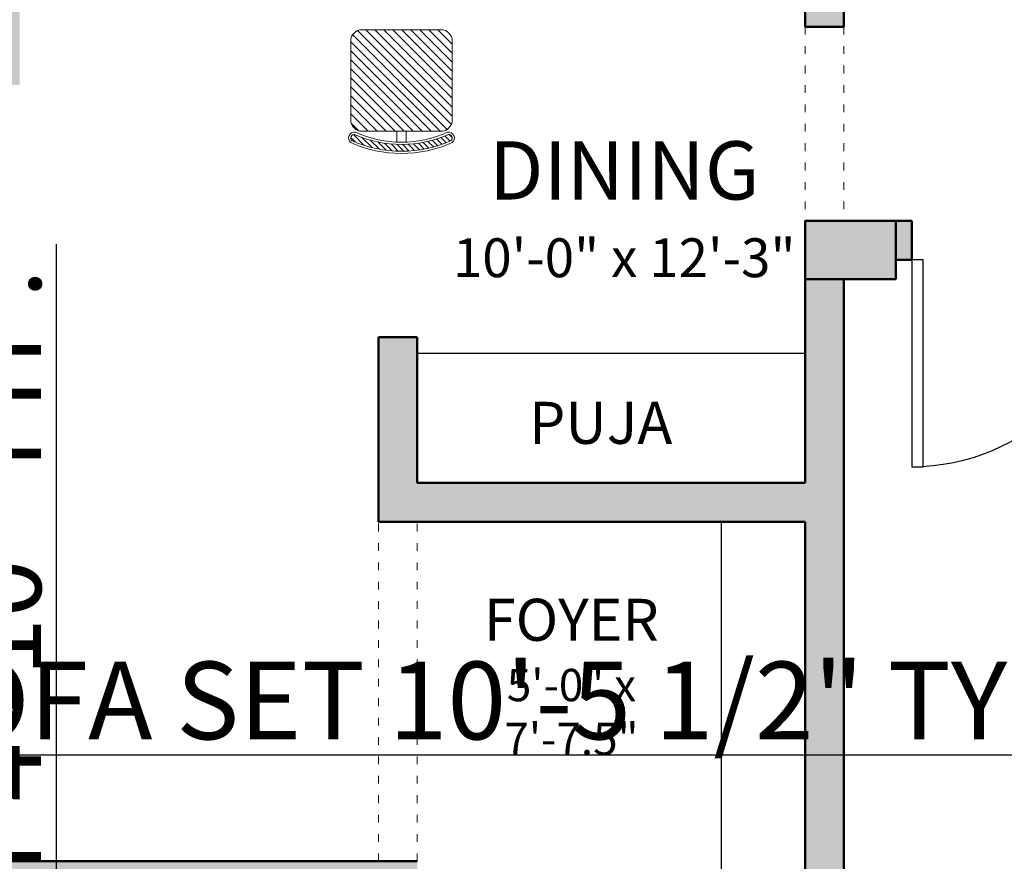
# Model space of a CAD drawing. Units: inches. Extents: x 375 to 1122, y 27 to 1069.
# Tile 83 of 155: x 667 to 819, y 716 to 846. Entities that reach past the tile are written whole.
import ezdxf

# ---------------------------------------------------------------- set-up
doc = ezdxf.new("R2010")
doc.units = ezdxf.units.IN
doc.linetypes.add('ACAD_ISO03W100', pattern=[30, 12, -18])
for name, color, linetype, lineweight in [('A-ANNO-DIMS', 2, 'Continuous', 18), ('A-AREA-IDEN', 7, 'Continuous', 18), ('A-COLS-PATT', 10, 'Continuous', 13), ('A-FLOR-MILL', 55, 'Continuous', 25), ('A-WALL-OVHD', 77, 'ACAD_ISO03W100', 18), ('A-WALL-PATT', 252, 'Continuous', 13), ('Columns', 10, 'Continuous', 50), ('Doors', 150, 'Continuous', 25), ('Furniture', 30, 'Continuous', 18), ('Walls', 250, 'Continuous', 50)]:
    doc.layers.add(name, color=color, linetype=linetype, lineweight=lineweight)
doc.styles.get("Standard").update_dxf_attribs({"font": 'arial.ttf'})
doc.dimstyles.new('ISO-25', dxfattribs={"dimtxt": 12, "dimasz": 2.5, "dimexe": 1.5, "dimexo": 1.5, "dimtad": 1, "dimdec": 1, "dimlunit": 3, "dimtxsty": 'Standard', "dimblk": 'ARCHTICK', "dimcen": 2.5, "dimadec": 0, "dimazin": 0, "dimtfac": 1, "dimtdec": 1, "dimtmove": 0, "dimatfit": 3, "dimfxl": 1.5, "dimfxlon": 1, "dimarcsym": 0})

# ---------------------------------------------------------------- blocks, each defined once
blk = doc.blocks.new('*U2')
for p, q in [((0, 0), (0, 4)), ((32, 0), (32, 4))]:
    blk.add_line(p, q)
blk.add_lwpolyline([(0, 0), (0, -32), (1.75, -32), (1.75, 0)], close=True)
blk.add_arc((0, 0), 32, 270, 0)
blk = doc.blocks.new('A$C403C54AD')
at = {"ltscale": 0.05}
for p, q in [((2.6911, 1.212, -0.0006), (2.3564, 0.8773, -0.0006)), ((2.6563, 1.212, -0.0006), (2.3564, 0.9121, -0.0006)), ((2.6215, 1.212, -0.0006), (2.3564, 0.9469, -0.0006)), ((2.5866, 1.212, -0.0006), (2.3564, 0.9818, -0.0006)), ((2.5518, 1.212, -0.0006), (2.3564, 1.0166, -0.0006)), ((2.517, 1.212, -0.0006), (2.3564, 1.0514, -0.0006)), ((2.4821, 1.212, -0.0006), (2.3564, 1.0862, -0.0006)), ((2.4473, 1.212, -0.0006), (2.3564, 1.1211, -0.0006)), ((2.4125, 1.212, -0.0006), (2.3564, 1.1559, -0.0006)), ((2.7225, 1.2085, -0.0006), (2.3599, 0.8459, -0.0006)), ((2.7416, 1.1928, -0.0006), (2.3756, 0.8268, -0.0006)), ((2.7734, 1.2115, -0.0006), (2.7615, 1.1996, -0.0006)), ((2.787, 1.2034, -0.0006), (2.767, 1.1834, -0.0006)), ((2.7934, 1.188, -0.0006), (2.7731, 1.1677, -0.0006)), ((2.7491, 1.1655, -0.0006), (2.4029, 0.8193, -0.0006)), ((2.7993, 1.1722, -0.0006), (2.7787, 1.1515, -0.0006)), ((2.8048, 1.1558, -0.0006), (2.7837, 1.1348, -0.0006)), ((2.7491, 1.1306, -0.0006), (2.4378, 0.8193, -0.0006)), ((2.8097, 1.139, -0.0006), (2.7882, 1.1175, -0.0006)), ((2.8141, 1.1216, -0.0006), (2.792, 1.0996, -0.0006)), ((2.7491, 1.0958, -0.0006), (2.4726, 0.8193, -0.0006)), ((2.8179, 1.1037, -0.0006), (2.7952, 1.081, -0.0006)), ((2.8211, 1.0851, -0.0006), (2.7977, 1.0617, -0.0006)), ((2.7491, 1.061, -0.0006), (2.5074, 0.8193, -0.0006)), ((2.8236, 1.0658, -0.0006), (2.7993, 1.0415, -0.0006)), ((2.8253, 1.0457, -0.0006), (2.8, 1.0205, -0.0006)), ((2.7491, 1.0262, -0.0006), (2.5422, 0.8193, -0.0006)), ((2.7491, 0.9913, -0.0006), (2.5771, 0.8193, -0.0006)), ((2.8261, 1.003, -0.0006), (2.7982, 0.9751, -0.0006)), ((2.8262, 1.0248, -0.0006), (2.7997, 0.9984, -0.0006)), ((2.7491, 0.9565, -0.0006), (2.6119, 0.8193, -0.0006)), ((2.8224, 0.9558, -0.0006), (2.7904, 0.9238, -0.0006)), ((2.8249, 0.98, -0.0006), (2.7952, 0.9504, -0.0006)), ((2.7491, 0.9217, -0.0006), (2.6467, 0.8193, -0.0006)), ((2.8184, 0.93, -0.0006), (2.7833, 0.8949, -0.0006)), ((2.7491, 0.8868, -0.0006), (2.6815, 0.8193, -0.0006)), ((2.8123, 0.9022, -0.0006), (2.7728, 0.8626, -0.0006)), ((2.7472, 0.8501, -0.0006), (2.7183, 0.8212, -0.0006)), ((2.8036, 0.8717, -0.0006), (2.7618, 0.8298, -0.0006)), ((2.791, 0.8373, -0.0006), (2.7733, 0.8196, -0.0006))]:
    blk.add_line(p, q, dxfattribs=at)
for p, q in [((2.7055, 1.212, -0.0006), (2.4001, 1.212, -0.0006)), ((2.3564, 1.1683, -0.0006), (2.3564, 0.8629, -0.0006)), ((2.7491, 0.8629, -0.0006), (2.7491, 1.1683, -0.0006)), ((2.7491, 1.0331, -0.0006), (2.7913, 1.0331, -0.0006)), ((2.7491, 0.9982, -0.0006), (2.7913, 0.9982, -0.0006)), ((2.4001, 0.8193, -0.0006), (2.531, 0.8193, -0.0006)), ((2.531, 0.8193, -0.0006), (2.7055, 0.8193, -0.0006))]:
    blk.add_line(p, q)
for centre, radius, start, end in [((2.7752, 1.1978, -0.0006), 0.0225, 38.8964, 189.6684), ((2.4001, 1.1683, -0.0006), 0.0436, 90, 180), ((2.7055, 1.1683, -0.0006), 0.0436, 0, 90), ((2.3575, 1.0156, -0.0006), 0.4338, 335.7176, 24.2824), ((2.3575, 1.0156, -0.0006), 0.4425, 335.7176, 24.2824), ((2.7752, 1.1978, -0.0006), 0.0138, 38.8964, 189.6684), ((2.3575, 1.0156, -0.0006), 0.4687, 335.7176, 24.2824), ((2.3575, 1.0156, -0.0006), 0.4774, 335.7176, 24.2824), ((2.4001, 0.8629, -0.0006), 0.0436, 180, 270), ((2.7055, 0.8629, -0.0006), 0.0436, 270, 0), ((2.7751, 0.8332, -0.0006), 0.0225, 169.7658, 321.6694), ((2.7751, 0.8332, -0.0006), 0.0138, 169.7658, 321.6694)]:
    blk.add_arc(centre, radius, start, end)
blk = doc.blocks.new('COLUMN-14X9IN')
blk.add_lwpolyline([(0, 0), (14, 0), (14, 9), (0, 9)], close=True)
blk = doc.blocks.new('_ArchTick')
at = {"color": 0, "linetype": 'ByBlock', "const_width": 0.15}
blk.add_lwpolyline([(-0.5, -0.5), (0.5, 0.5)], dxfattribs=at)
blk = doc.blocks.new('*D57')
at = {"layer": 'A-ANNO-DIMS', "color": 0, "lineweight": -2, "transparency": 16777216}
for p, q in [((512.46, 733.49), (512.46, 730.49)), ((638.07, 733.49), (638.07, 730.49)), ((512.46, 731.99), (638.07, 731.99)), ((638.07, 731.99), (839.76, 731.99))]:
    blk.add_line(p, q, dxfattribs=at)
at = {"layer": 'Defpoints', "color": 0, "transparency": 16777216}
for p in [(512.46, 750.84), (638.07, 750.84), (638.07, 731.99)]:
    blk.add_point(p, dxfattribs=at)
at = {"layer": 'A-ANNO-DIMS', "color": 0, "lineweight": -2, "transparency": 16777216, "xscale": 2.5, "yscale": 2.5, "zscale": 2.5, "rotation": 180}
blk.add_blockref('_ArchTick', (512.46, 731.99), dxfattribs=at)
at = {"layer": 'A-ANNO-DIMS', "color": 0, "lineweight": -2, "transparency": 16777216, "xscale": 2.5, "yscale": 2.5, "zscale": 2.5}
blk.add_blockref('_ArchTick', (638.07, 731.99), dxfattribs=at)
at = {"layer": 'A-ANNO-DIMS', "color": 0, "transparency": 16777216, "insert": (740.16, 738.83), "char_height": 12, "attachment_point": 5}
blk.add_mtext('SOFA SET 10\'-5 1/2" TYP.', dxfattribs=at)
blk = doc.blocks.new('*D58')
at = {"layer": 'A-ANNO-DIMS', "color": 0, "lineweight": -2, "transparency": 16777216}
for p, q in [((656.91, 835.53), (656.91, 940.29)), ((655.41, 835.53), (658.41, 835.53)), ((656.91, 750.84), (656.91, 835.53)), ((655.41, 750.84), (658.41, 750.84))]:
    blk.add_line(p, q, dxfattribs=at)
at = {"layer": 'Defpoints', "color": 0, "transparency": 16777216}
for p in [(638.07, 835.53), (656.91, 835.53), (638.07, 750.84)]:
    blk.add_point(p, dxfattribs=at)
at = {"layer": 'A-ANNO-DIMS', "color": 0, "lineweight": -2, "transparency": 16777216, "xscale": 2.5, "yscale": 2.5, "zscale": 2.5}
for p, rotation in [((656.91, 835.53), 90), ((656.91, 750.84), 270)]:
    blk.add_blockref('_ArchTick', p, dxfattribs=dict(at, rotation=rotation))
at = {"layer": 'A-ANNO-DIMS', "color": 0, "transparency": 16777216, "insert": (650.08, 889.16), "char_height": 12, "attachment_point": 5, "rotation": 90}
blk.add_mtext('7\'-0 1/2" TYP.', dxfattribs=at)
blk = doc.blocks.new('*D79')
at = {"layer": 'A-ANNO-DIMS', "color": 0, "lineweight": -2, "transparency": 16777216}
for p, q in [((672.21, 647.53), (672.21, 810.92)), ((670.71, 647.53), (673.71, 647.53)), ((672.21, 589.53), (672.21, 647.53)), ((670.71, 589.53), (673.71, 589.53))]:
    blk.add_line(p, q, dxfattribs=at)
at = {"layer": 'Defpoints', "color": 0, "transparency": 16777216}
for p in [(663.51, 647.53), (672.21, 647.53), (663.51, 589.53)]:
    blk.add_point(p, dxfattribs=at)
at = {"layer": 'A-ANNO-DIMS', "color": 0, "lineweight": -2, "transparency": 16777216, "xscale": 2.5, "yscale": 2.5, "zscale": 2.5}
for p, rotation in [((672.21, 647.53), 90), ((672.21, 589.53), 270)]:
    blk.add_blockref('_ArchTick', p, dxfattribs=dict(at, rotation=rotation))
at = {"layer": 'A-ANNO-DIMS', "color": 0, "transparency": 16777216, "insert": (665.38, 730.47), "char_height": 12, "attachment_point": 5, "rotation": 90}
blk.add_mtext('CABINET 4\'-10" TYP.', dxfattribs=at)
blk = doc.blocks.new('*D85')
at = {"layer": 'A-ANNO-DIMS', "color": 0, "lineweight": -2, "transparency": 16777216}
for p, q in [((401.51, 868.53), (398.51, 868.53)), ((400.01, 814.53), (400.01, 868.53)), ((401.51, 814.53), (398.51, 814.53))]:
    blk.add_line(p, q, dxfattribs=at)
at = {"layer": 'Defpoints', "color": 0, "transparency": 16777216}
for p in [(400.01, 868.53), (845.01, 868.53), (845.01, 814.53)]:
    blk.add_point(p, dxfattribs=at)
at = {"layer": 'A-ANNO-DIMS', "color": 0, "lineweight": -2, "transparency": 16777216, "xscale": 2.5, "yscale": 2.5, "zscale": 2.5}
for p, rotation in [((400.01, 868.53), 90), ((400.01, 814.53), 270)]:
    blk.add_blockref('_ArchTick', p, dxfattribs=dict(at, rotation=rotation))
at = {"layer": 'A-ANNO-DIMS', "color": 0, "transparency": 16777216, "insert": (393.26, 841.53), "char_height": 12, "attachment_point": 5, "rotation": 90}
blk.add_mtext('4\'-6"', dxfattribs=at)
blk = doc.blocks.new('*D88')
at = {"layer": 'A-ANNO-DIMS', "color": 0, "lineweight": -2, "transparency": 16777216}
for p, q in [((731.01, 1052.53), (731.01, 1055.53)), ((854.01, 1052.53), (854.01, 1055.53)), ((731.01, 1054.03), (854.01, 1054.03))]:
    blk.add_line(p, q, dxfattribs=at)
at = {"layer": 'Defpoints', "color": 0, "transparency": 16777216}
for p in [(854.01, 1054.03), (731.01, 502.53), (854.01, 502.53)]:
    blk.add_point(p, dxfattribs=at)
at = {"layer": 'A-ANNO-DIMS', "color": 0, "lineweight": -2, "transparency": 16777216, "xscale": 2.5, "yscale": 2.5, "zscale": 2.5, "rotation": 180}
blk.add_blockref('_ArchTick', (731.01, 1054.03), dxfattribs=at)
at = {"layer": 'A-ANNO-DIMS', "color": 0, "lineweight": -2, "transparency": 16777216, "xscale": 2.5, "yscale": 2.5, "zscale": 2.5}
blk.add_blockref('_ArchTick', (854.01, 1054.03), dxfattribs=at)
at = {"layer": 'A-ANNO-DIMS', "color": 0, "transparency": 16777216, "insert": (792.51, 1060.78), "char_height": 12, "attachment_point": 5}
blk.add_mtext('10\'-3"', dxfattribs=at)
blk = doc.blocks.new('*D91')
at = {"layer": 'A-ANNO-DIMS', "color": 0, "lineweight": -2, "transparency": 16777216}
for p, q in [((728.01, 1052.53), (728.01, 1055.53)), ((788.01, 1052.53), (788.01, 1055.53)), ((728.01, 1054.03), (788.01, 1054.03))]:
    blk.add_line(p, q, dxfattribs=at)
at = {"layer": 'Defpoints', "color": 0, "transparency": 16777216}
for p in [(788.01, 1054.03), (728.01, 774.03), (788.01, 774.03)]:
    blk.add_point(p, dxfattribs=at)
at = {"layer": 'A-ANNO-DIMS', "color": 0, "lineweight": -2, "transparency": 16777216, "xscale": 2.5, "yscale": 2.5, "zscale": 2.5, "rotation": 180}
blk.add_blockref('_ArchTick', (728.01, 1054.03), dxfattribs=at)
at = {"layer": 'A-ANNO-DIMS', "color": 0, "lineweight": -2, "transparency": 16777216, "xscale": 2.5, "yscale": 2.5, "zscale": 2.5}
blk.add_blockref('_ArchTick', (788.01, 1054.03), dxfattribs=at)
at = {"layer": 'A-ANNO-DIMS', "color": 0, "transparency": 16777216, "insert": (758.01, 1060.78), "char_height": 12, "attachment_point": 5}
blk.add_mtext('5\'-0"', dxfattribs=at)

msp = doc.modelspace()

# ---------------------------------------------------------------- hatches: boundary and pattern name
at = {"layer": 'A-COLS-PATT'}
h = msp.add_hatch(color=256, dxfattribs=at)
h.dxf.hatch_style = 1
h.paths.add_polyline_path([(512.51, 982.53), (498.51, 982.53), (498.51, 973.53), (512.51, 973.53)])
h.paths.add_polyline_path([(666.51, 982.53), (652.51, 982.53), (652.51, 973.53), (666.51, 973.53)])
h.paths.add_polyline_path([(802.01, 982.53), (788.01, 982.53), (788.01, 973.53), (802.01, 973.53)])
h.paths.add_polyline_path([(932.01, 982.53), (918.01, 982.53), (918.01, 973.53), (932.01, 973.53)])
h.paths.add_polyline_path([(507.51, 841.53), (498.51, 841.53), (498.51, 827.53), (507.51, 827.53)])
h.paths.add_polyline_path([(666.51, 844.53), (652.51, 844.53), (652.51, 835.53), (666.51, 835.53)])
h.paths.add_polyline_path([(802.01, 814.53), (788.01, 814.53), (788.01, 805.53), (802.01, 805.53)])
h.paths.add_polyline_path([(932.01, 814.53), (918.01, 814.53), (918.01, 805.53), (932.01, 805.53)])
h.paths.add_polyline_path([(507.51, 719.53), (498.51, 719.53), (498.51, 705.53), (507.51, 705.53)])
h.paths.add_polyline_path([(731.01, 676.53), (722.01, 676.53), (722.01, 662.53), (731.01, 662.53)])
h.paths.add_polyline_path([(802.01, 676.53), (788.01, 676.53), (788.01, 667.53), (802.01, 667.53)])
h.paths.add_polyline_path([(932.01, 676.53), (918.01, 676.53), (918.01, 667.53), (932.01, 667.53)])
h.paths.add_polyline_path([(932.01, 583.53), (918.01, 583.53), (918.01, 574.53), (932.01, 574.53)])
h.paths.add_polyline_path([(868.01, 583.53), (854.01, 583.53), (854.01, 574.53), (868.01, 574.53)])
h.paths.add_polyline_path([(868.01, 502.53), (854.01, 502.53), (854.01, 493.53), (868.01, 493.53)])
h.paths.add_polyline_path([(932.01, 502.53), (918.01, 502.53), (918.01, 493.53), (932.01, 493.53)])
h.paths.add_polyline_path([(672.51, 592.03), (663.51, 592.03), (663.51, 578.03), (672.51, 578.03)])
h.paths.add_polyline_path([(512.51, 589.53), (498.51, 589.53), (498.51, 580.53), (512.51, 580.53)])
h.paths.add_polyline_path([(507.51, 464.53), (498.51, 464.53), (498.51, 450.53), (507.51, 450.53)])
h.paths.add_polyline_path([(731.01, 507.53), (722.01, 507.53), (722.01, 493.53), (731.01, 493.53)])
h.paths.add_polyline_path([(802.01, 502.53), (788.01, 502.53), (788.01, 493.53), (802.01, 493.53)])
h.paths.add_polyline_path([(507.51, 342.53), (498.51, 342.53), (498.51, 328.53), (507.51, 328.53)])
h.paths.add_polyline_path([(512.51, 196.53), (498.51, 196.53), (498.51, 187.53), (512.51, 187.53)])
h.paths.add_polyline_path([(666.51, 334.53), (652.51, 334.53), (652.51, 325.53), (666.51, 325.53)])
h.paths.add_polyline_path([(666.51, 196.53), (652.51, 196.53), (652.51, 187.53), (666.51, 187.53)])
h.paths.add_polyline_path([(805.01, 196.53), (791.01, 196.53), (791.01, 187.53), (805.01, 187.53)])
h.paths.add_polyline_path([(932.01, 196.53), (918.01, 196.53), (918.01, 187.53), (932.01, 187.53)])
h.paths.add_polyline_path([(932.01, 334.53), (918.01, 334.53), (918.01, 325.53), (932.01, 325.53)])
h.paths.add_polyline_path([(805.01, 334.53), (791.01, 334.53), (791.01, 325.53), (805.01, 325.53)])
at = {"layer": 'A-WALL-PATT'}
h = msp.add_hatch(color=256, dxfattribs=at)
h.dxf.hatch_style = 1
h.paths.add_polyline_path([(962.01, 388.53), (989.01, 388.53), (989.01, 394.53), (962.01, 394.53), (932.01, 394.53), (932.01, 397.53), (923.01, 397.53), (923.01, 394.53), (842.01, 394.53), (842.01, 334.53), (839.51, 334.53), (839.51, 328.53), (854.01, 328.53), (854.01, 334.53), (848.01, 334.53), (848.01, 388.53), (953.01, 388.53), (953.01, 356.08), (962.01, 356.08), (962.01, 358.55), (989.01, 358.55), (989.01, 364.55), (962.01, 364.55)])
h.paths.add_polyline_path([(989.01, 502.53), (932.01, 502.53), (932.01, 583.53), (932.01, 593.53), (923.01, 593.53), (923.01, 583.53), (854.01, 583.53), (854.01, 556.53), (863.01, 556.53), (863.01, 574.53), (923.01, 574.53), (923.01, 502.53), (863.01, 502.53), (863.01, 520.53), (854.01, 520.53), (854.01, 502.53), (773.01, 502.53), (773.01, 493.53), (788.01, 493.53), (788.01, 402.03), (722.01, 402.03), (722.01, 373.53), (728.01, 373.53), (728.01, 396.03), (788.01, 396.03), (788.01, 373.53), (794.01, 373.53), (794.01, 430.53), (814.01, 430.53), (814.01, 436.53), (794.01, 436.53), (794.01, 493.53), (923.01, 493.53), (923.01, 487.53), (932.01, 487.53), (932.01, 493.53), (983.01, 493.53), (983.01, 473.53), (989.01, 473.53)])
h.paths.add_polyline_path([(797.01, 325.53), (805.01, 325.53), (805.01, 328.53), (807.51, 328.53), (807.51, 334.53), (791.01, 334.53), (791.01, 226.53), (770.76, 226.53), (770.76, 217.53), (791.01, 217.53), (791.01, 187.53), (855.01, 187.53), (855.01, 196.53), (797.01, 196.53)])
h.paths.add_polyline_path([(989.01, 238.53), (962.01, 238.53), (962.01, 256.42), (953.01, 256.42), (953.01, 229.53), (980.01, 229.53), (980.01, 196.53), (915.01, 196.53), (915.01, 187.53), (989.01, 187.53)])
h.paths.add_polyline_path([(962.01, 334.53), (884.01, 334.53), (884.01, 328.53), (918.01, 328.53), (918.01, 325.53), (932.01, 325.53), (932.01, 328.53), (953.01, 328.53), (953.01, 304.42), (962.01, 304.42)])
h.paths.add_polyline_path([(606.51, 283.53), (609.51, 283.53), (609.51, 289.53), (600.51, 289.53), (600.51, 196.53), (578.51, 196.53), (578.51, 187.53), (606.51, 187.53), (606.51, 196.53)])
h.paths.add_polyline_path([(666.51, 292.53), (660.51, 292.53), (660.51, 289.53), (633.51, 289.53), (633.51, 283.53), (660.51, 283.53), (660.51, 196.53), (628.01, 196.53), (628.01, 187.53), (630.53, 187.53), (630.53, 160.53), (636.53, 160.53), (636.53, 187.53), (660.51, 187.53), (660.51, 160.53), (666.51, 160.53), (666.51, 217.53), (686.76, 217.53), (686.76, 226.53), (666.51, 226.53)])
h.paths.add_polyline_path([(480.51, 256.42), (471.51, 256.42), (471.51, 238.53), (444.51, 238.53), (444.51, 187.53), (518.51, 187.53), (518.51, 196.53), (453.51, 196.53), (453.51, 229.53), (480.51, 229.53)])
h.paths.add_polyline_path([(480.51, 328.53), (652.51, 328.53), (652.51, 325.53), (660.51, 325.53), (660.51, 322.53), (666.51, 322.53), (666.51, 334.53), (507.51, 334.53), (507.51, 360.53), (498.51, 360.53), (498.51, 334.53), (471.51, 334.53), (471.51, 304.42), (480.51, 304.42)])
h.paths.add_polyline_path([(507.51, 484.53), (498.51, 484.53), (498.51, 444.53), (507.51, 444.53), (507.51, 454.53), (621.51, 454.53), (621.51, 460.53), (507.51, 460.53)])
h.paths.add_polyline_path([(672.51, 604.53), (683.26, 604.53), (683.26, 613.53), (669.51, 613.53), (669.51, 649.53), (663.51, 649.53), (663.51, 589.53), (507.51, 589.53), (507.51, 613.53), (498.51, 613.53), (498.51, 556.53), (507.51, 556.53), (507.51, 580.53), (663.51, 580.53), (663.51, 520.53), (669.51, 520.53), (669.51, 556.53), (683.26, 556.53), (683.26, 565.53), (672.51, 565.53)])
h.paths.add_polyline_path([(731.01, 667.53), (734.01, 667.53), (734.01, 676.53), (728.01, 676.53), (728.01, 715.53), (657.51, 715.53), (657.51, 709.53), (663.51, 709.53), (663.51, 673.53), (669.51, 673.53), (669.51, 709.53), (722.01, 709.53), (722.01, 613.53), (704.76, 613.53), (704.76, 604.53), (722.01, 604.53), (722.01, 565.53), (704.76, 565.53), (704.76, 556.53), (722.01, 556.53), (722.01, 502.53), (722.01, 460.53), (669.51, 460.53), (669.51, 496.53), (663.51, 496.53), (663.51, 460.53), (657.51, 460.53), (657.51, 454.53), (728.01, 454.53), (728.01, 493.53), (734.01, 493.53), (734.01, 502.53), (731.01, 502.53)])
h.paths.add_polyline_path([(986.01, 718.53), (959.01, 718.53), (959.01, 727.53), (950.01, 727.53), (950.01, 709.53), (977.01, 709.53), (977.01, 676.53), (794.01, 676.53), (794.01, 805.53), (802.01, 805.53), (802.01, 808.53), (804.51, 808.53), (804.51, 814.53), (788.01, 814.53), (788.01, 774.03), (728.01, 774.03), (728.01, 796.53), (722.01, 796.53), (722.01, 768.03), (788.01, 768.03), (788.01, 676.53), (773.01, 676.53), (773.01, 667.53), (923.01, 667.53), (923.01, 657.53), (932.01, 657.53), (932.01, 667.53), (986.01, 667.53)])
h.paths.add_polyline_path([(621.51, 715.53), (507.51, 715.53), (507.51, 733.53), (498.51, 733.53), (498.51, 715.53), (498.51, 685.53), (507.51, 685.53), (507.51, 709.53), (621.51, 709.53)])
h.paths.add_polyline_path([(666.51, 847.03), (660.51, 847.03), (660.51, 844.53), (652.51, 844.53), (652.51, 841.53), (480.51, 841.53), (480.51, 859.53), (471.51, 859.53), (471.51, 835.53), (498.51, 835.53), (498.51, 817.53), (507.51, 817.53), (507.51, 835.53), (666.51, 835.53)])
h.paths.add_polyline_path([(480.51, 940.53), (453.51, 940.53), (453.51, 973.53), (518.51, 973.53), (518.51, 982.53), (444.51, 982.53), (444.51, 931.53), (471.51, 931.53), (471.51, 907.53), (480.51, 907.53)])
h.paths.add_polyline_path([(606.51, 982.53), (578.51, 982.53), (578.51, 973.53), (600.51, 973.53), (600.51, 880.53), (609.51, 880.53), (609.51, 886.53), (606.51, 886.53)])
h.paths.add_polyline_path([(666.51, 943.53), (686.76, 943.53), (686.76, 952.53), (666.51, 952.53), (666.51, 1009.53), (660.51, 1009.53), (660.51, 982.53), (636.53, 982.53), (636.53, 1009.53), (630.53, 1009.53), (630.53, 982.53), (628.01, 982.53), (628.01, 973.53), (660.51, 973.53), (660.51, 886.53), (633.51, 886.53), (633.51, 880.53), (660.51, 880.53), (660.51, 877.03), (666.51, 877.03)])
h.paths.add_polyline_path([(986.01, 874.53), (932.01, 874.53), (932.01, 877.53), (923.01, 877.53), (923.01, 874.53), (788.01, 874.53), (788.01, 868.53), (788.01, 844.53), (794.01, 844.53), (794.01, 868.53), (839.01, 868.53), (839.01, 814.53), (836.51, 814.53), (836.51, 808.53), (851.01, 808.53), (851.01, 814.53), (845.01, 814.53), (845.01, 868.53), (986.01, 868.53)])
h.paths.add_polyline_path([(959.01, 838.55), (986.01, 838.55), (986.01, 844.55), (959.01, 844.55), (959.01, 847.03), (950.01, 847.03), (950.01, 814.53), (881.01, 814.53), (881.01, 808.53), (918.01, 808.53), (918.01, 805.53), (932.01, 805.53), (932.01, 808.53), (950.01, 808.53), (950.01, 793.53), (959.01, 793.53)])
h.paths.add_polyline_path([(986.01, 982.53), (899.01, 982.53), (899.01, 973.53), (923.01, 973.53), (923.01, 967.53), (932.01, 967.53), (932.01, 973.53), (980.01, 973.53), (980.01, 953.53), (986.01, 953.53)])
h.paths.add_polyline_path([(851.01, 982.53), (788.01, 982.53), (788.01, 952.53), (770.76, 952.53), (770.76, 943.53), (788.01, 943.53), (788.01, 910.53), (814.01, 910.53), (814.01, 916.53), (794.01, 916.53), (794.01, 973.53), (851.01, 973.53)])

# ---------------------------------------------------------------- linework, layer by layer
at = {"layer": 'A-FLOR-MILL'}
for p, q in [((788.01, 794.03), (728.01, 794.03)), ((775.01, 768.03), (775.01, 676.53))]:
    msp.add_line(p, q, dxfattribs=at)
at = {"layer": 'A-WALL-OVHD', "ltscale": 0.1}
for p, q in [((788.01, 844.53), (788.01, 814.53)), ((794.01, 844.53), (794.01, 814.53)), ((722.01, 715.53), (722.01, 768.03)), ((728.01, 715.53), (728.01, 768.03))]:
    msp.add_line(p, q, dxfattribs=at)
at = {"layer": 'Walls'}
for p, q in [((788.01, 868.53), (788.01, 844.53)), ((794.01, 844.53), (794.01, 868.53)), ((794.01, 844.53), (788.01, 844.53)), ((788.01, 814.53), (804.51, 814.53)), ((788.01, 814.53), (788.01, 774.03)), ((804.51, 814.53), (804.51, 808.53)), ((802.01, 805.53), (802.01, 808.53)), ((802.01, 808.53), (804.51, 808.53)), ((794.01, 805.53), (794.01, 676.53)), ((794.01, 805.53), (802.01, 805.53)), ((722.01, 796.53), (722.01, 768.03)), ((722.01, 796.53), (728.01, 796.53)), ((728.01, 796.53), (728.01, 774.03)), ((788.01, 774.03), (728.01, 774.03)), ((788.01, 768.03), (722.01, 768.03)), ((788.01, 768.03), (788.01, 676.53)), ((657.51, 715.53), (728.01, 715.53))]:
    msp.add_line(p, q, dxfattribs=at)

# ---------------------------------------------------------------- block references
at = {"layer": 'Columns'}
msp.add_blockref('COLUMN-14X9IN', (788.01, 805.53), dxfattribs=at)
at = {"layer": 'Doors'}
msp.add_blockref('*U2', (804.51, 808.53), dxfattribs=at)
at = {"layer": 'Furniture', "xscale": 39.9918517141215, "yscale": 39.9918517141215, "zscale": 39.9918517141215, "rotation": 270}
msp.add_blockref('A$C403C54AD', (684.95, 938.32, 0.02), dxfattribs=at)

# ---------------------------------------------------------------- texts
at = {"layer": 'A-AREA-IDEN', "attachment_point": 7}
for s, width, insert, char_height in [('\\pxqc;{\\fArial|b1|i0|c0|p34;\\H0.75x;DINING\\H1.33333x;\\P\\fArial|b0|i0|c0|p34;\\H0.5x;10\'-0" x 12\'-3"}', 66.1169, (726.96, 805.83), 12), ('\\pxqc;{\\fArial|b1|i0|c0|p34;PUJA}', 42.2291, (735.26, 780.06), 6.5), ('\\pxqc;{\\fArial|b1|i0|c0|p34;FOYER\\P\\fArial|b0|i0|c0|p34;\\H0.76923x;5\'-0" x 7\'-7.5"}', 42.2291, (730.74, 731.94), 6.5)]:
    msp.add_mtext_dynamic_manual_height_columns(s, width=width, gutter_width=12.5, heights=[0], dxfattribs=dict(at, insert=insert, char_height=char_height))

# ---------------------------------------------------------------- dimensions: what is measured, and where the dimension line sits
at = {"layer": 'A-ANNO-DIMS'}
for base, p1, p2, picture, middle in [((788.01, 1054.03), (728.01, 774.03), (788.01, 774.03), '*D91', (758.01, 1060.78)), ((854.01, 1054.03), (731.01, 502.53), (854.01, 502.53), '*D88', (792.51, 1060.78))]:
    dim = msp.add_linear_dim(base=base, p1=p1, p2=p2, dimstyle='ISO-25', override={"dimdec": 1, "dimlfac": 1, "dimrnd": 0, "dimzin": 1, "dimdsep": 46, "dimlunit": 4, "dimfrac": 2}, dxfattribs=at)
    dim.commit()
    dim.dimension.update_dxf_attribs({"geometry": picture, "text_midpoint": middle})
for base, p1, p2, text, picture, middle in [((656.91, 835.53), (638.07, 750.84), (638.07, 835.53), '<> TYP.', '*D58', (650.08, 889.16)), ((672.21, 647.53), (663.51, 589.53), (663.51, 647.53), 'CABINET <> TYP.', '*D79', (665.38, 730.47))]:
    dim = msp.add_linear_dim(base=base, p1=p1, p2=p2, angle=90, text=text, dimstyle='ISO-25', override={"dimdec": 1, "dimlfac": 1, "dimrnd": 0, "dimzin": 1, "dimdsep": 46, "dimlunit": 4, "dimfrac": 2}, dxfattribs=at)
    dim.commit()
    dim.dimension.update_dxf_attribs({"geometry": picture, "text_midpoint": middle})
dim = msp.add_linear_dim(base=(400.01, 868.53), p1=(845.01, 814.53), p2=(845.01, 868.53), angle=90, dimstyle='ISO-25', override={"dimdec": 1, "dimlfac": 1, "dimrnd": 0, "dimzin": 1, "dimdsep": 46, "dimlunit": 4, "dimfrac": 2}, dxfattribs=at)
dim.commit()
dim.dimension.update_dxf_attribs({"geometry": '*D85', "text_midpoint": (393.26, 841.53)})
dim = msp.add_linear_dim(base=(638.07, 731.99), p1=(512.46, 750.84), p2=(638.07, 750.84), text='SOFA SET <> TYP.', dimstyle='ISO-25', override={"dimdec": 1, "dimlfac": 1, "dimrnd": 0, "dimzin": 1, "dimdsep": 46, "dimlunit": 4, "dimfrac": 2}, dxfattribs=at)
dim.commit()
dim.dimension.update_dxf_attribs({"geometry": '*D57', "text_midpoint": (740.16, 738.83)})

doc.saveas('drawing.dxf')
